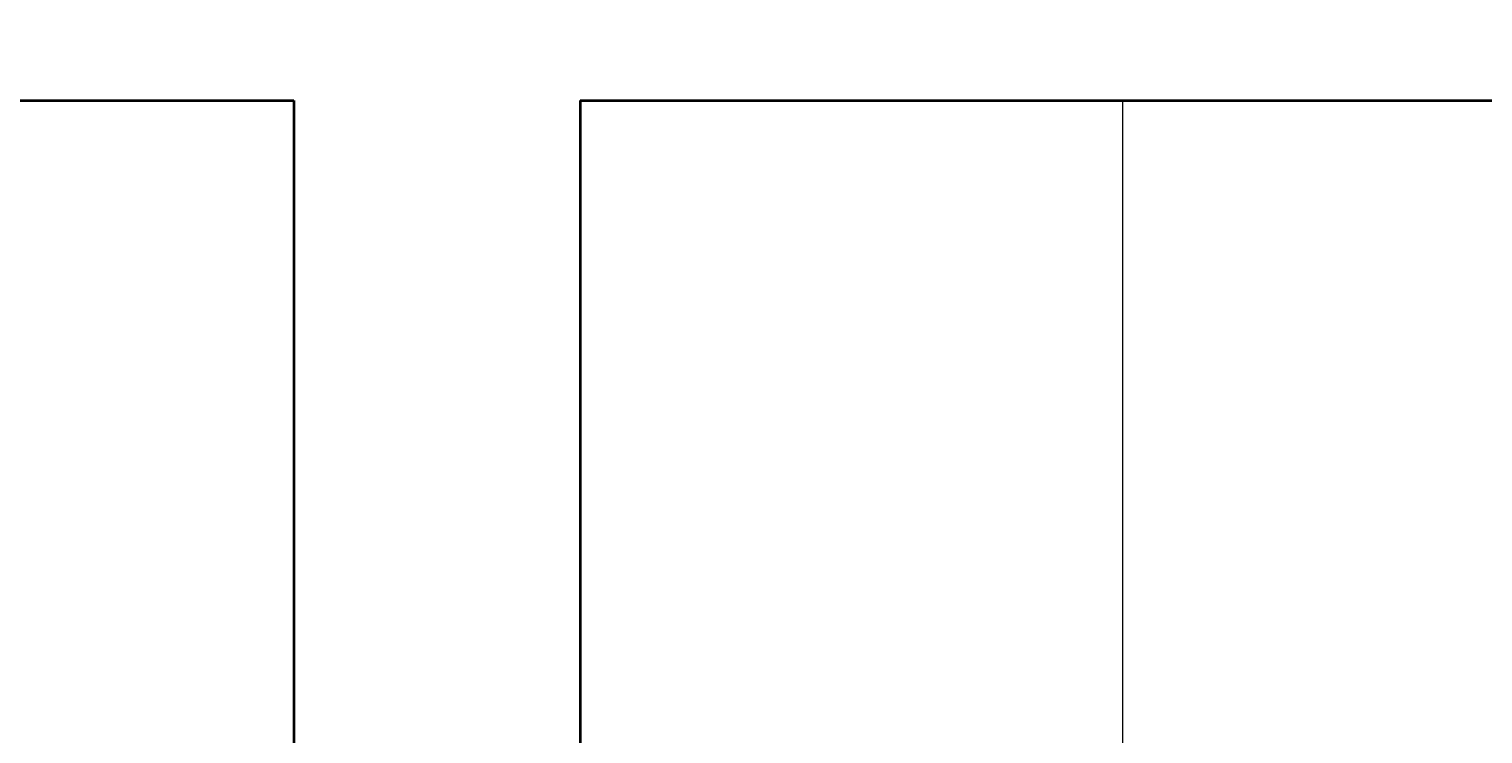
# Model space of a CAD drawing. Units: millimetres. Extents: x 27017497 to 27018854, y 7058029 to 7059154.
# Tile 17 of 91: x 27017605 to 27017651, y 7058275 to 7058297. Entities that reach past the tile are written whole.
import ezdxf

# ---------------------------------------------------------------- set-up
doc = ezdxf.new("R2010")
doc.units = ezdxf.units.MM
for name, color, linetype, lineweight in [('A-ANNO-DIMS', 2, 'Continuous', 18), ('A-FLOR-CASE', 8, 'Continuous', 20), ('A-WALL', 7, 'Continuous', 35)]:
    doc.layers.add(name, color=color, linetype=linetype, lineweight=lineweight)
doc.styles.get("Standard").update_dxf_attribs({"font": 'arial.ttf'})
doc.dimstyles.get("Standard").update_dxf_attribs({"dimtxt": 0.18, "dimasz": 0.18, "dimexe": 0.18, "dimexo": 0.0625, "dimgap": 0.09, "dimtad": 0, "dimtih": 1, "dimtoh": 1, "dimdec": 4, "dimzin": 0, "dimdsep": 46, "dimtxsty": 'Standard', "dimcen": 0.09, "dimadec": 0, "dimazin": 0, "dimtfac": 1, "dimtdec": 4, "dimtofl": 0, "dimtmove": 0, "dimatfit": 3, "dimfxl": 1, "dimtolj": 1, "dimtzin": 0, "dimarcsym": 0})

# ---------------------------------------------------------------- blocks, each defined once
blk = doc.blocks.new('*D47')
at = {"layer": 'A-ANNO-DIMS', "color": 0, "lineweight": -2, "transparency": 16777216}
for p, q in [((27017561.166, 7058294.35), (27017561.166, 7058028.6)), ((27018790.606, 7058294.35), (27018790.606, 7058028.6)), ((27017561.346, 7058028.78), (27018175.431, 7058028.78)), ((27018790.426, 7058028.78), (27018176.341, 7058028.78))]:
    blk.add_line(p, q, dxfattribs=at)
at = {"layer": 'A-ANNO-DIMS', "color": 0, "transparency": 16777216}
for points in [[(27017561.346, 7058028.81), (27017561.346, 7058028.75), (27017561.166, 7058028.78)], [(27018790.426, 7058028.81), (27018790.426, 7058028.75), (27018790.606, 7058028.78)]]:
    blk.add_solid(points, dxfattribs=at)
at = {"layer": 'Defpoints', "color": 0, "transparency": 16777216}
for p in [(27017561.166, 7058294.412), (27018790.606, 7058294.412), (27018790.606, 7058028.78)]:
    blk.add_point(p, dxfattribs=at)
at = {"layer": 'A-ANNO-DIMS', "color": 0, "transparency": 16777216, "insert": (27018175.886, 7058028.78), "char_height": 0.18, "attachment_point": 5}
blk.add_mtext('\\A1;1229.4', dxfattribs=at)
blk = doc.blocks.new('*D48')
at = {"layer": 'A-ANNO-DIMS', "color": 0, "lineweight": -2, "transparency": 16777216}
for p, q in [((27018463.498, 7058622.912), (27017497.536, 7058622.912)), ((27017497.716, 7058622.732), (27017497.716, 7058357.753)), ((27017497.716, 7058092.41), (27017497.716, 7058357.389)), ((27018555.129, 7058092.23), (27017497.536, 7058092.23))]:
    blk.add_line(p, q, dxfattribs=at)
at = {"layer": 'A-ANNO-DIMS', "color": 0, "transparency": 16777216}
for points in [[(27017497.686, 7058622.732), (27017497.746, 7058622.732), (27017497.716, 7058622.912)], [(27017497.686, 7058092.41), (27017497.746, 7058092.41), (27017497.716, 7058092.23)]]:
    blk.add_solid(points, dxfattribs=at)
at = {"layer": 'Defpoints', "color": 0, "transparency": 16777216}
for p in [(27018463.561, 7058622.912), (27017497.716, 7058092.23), (27018555.192, 7058092.23)]:
    blk.add_point(p, dxfattribs=at)
at = {"layer": 'A-ANNO-DIMS', "color": 0, "transparency": 16777216, "insert": (27017497.716, 7058357.571), "char_height": 0.18, "attachment_point": 5}
blk.add_mtext('\\A1;530.7', dxfattribs=at)

msp = doc.modelspace()

# ---------------------------------------------------------------- linework, layer by layer
at = {"layer": 'A-FLOR-CASE'}
msp.add_line((27017639.716, 7058294.412), (27017639.716, 7058207.055), dxfattribs=at)
at = {"layer": 'A-WALL'}
for p, q in [((27017561.166, 7058294.412), (27017613.666, 7058294.412)), ((27017613.666, 7058294.412), (27017613.666, 7058132.912)), ((27017622.666, 7058294.412), (27017622.666, 7058141.912)), ((27017622.666, 7058294.412), (27017758.765, 7058294.412))]:
    msp.add_line(p, q, dxfattribs=at)

# ---------------------------------------------------------------- dimensions: what is measured, and where the dimension line sits
at = {"layer": 'A-ANNO-DIMS'}
dim = msp.add_linear_dim(base=(27017497.716, 7058092.23), p1=(27018463.561, 7058622.912), p2=(27018555.192, 7058092.23), angle=90, dimstyle='Standard', override={"dimdec": 1, "dimlfac": 1, "dimrnd": 0, "dimzin": 0, "dimdsep": 46, "dimlunit": 2}, dxfattribs=at)
dim.commit()
dim.dimension.update_dxf_attribs({"geometry": '*D48', "text_midpoint": (27017497.716, 7058357.571)})
dim = msp.add_linear_dim(base=(27018790.606, 7058028.78), p1=(27017561.166, 7058294.412), p2=(27018790.606, 7058294.412), dimstyle='Standard', override={"dimdec": 1, "dimlfac": 1, "dimrnd": 0, "dimzin": 0, "dimdsep": 46, "dimlunit": 2}, dxfattribs=at)
dim.commit()
dim.dimension.update_dxf_attribs({"geometry": '*D47', "text_midpoint": (27018175.886, 7058028.78)})

doc.saveas('drawing.dxf')
